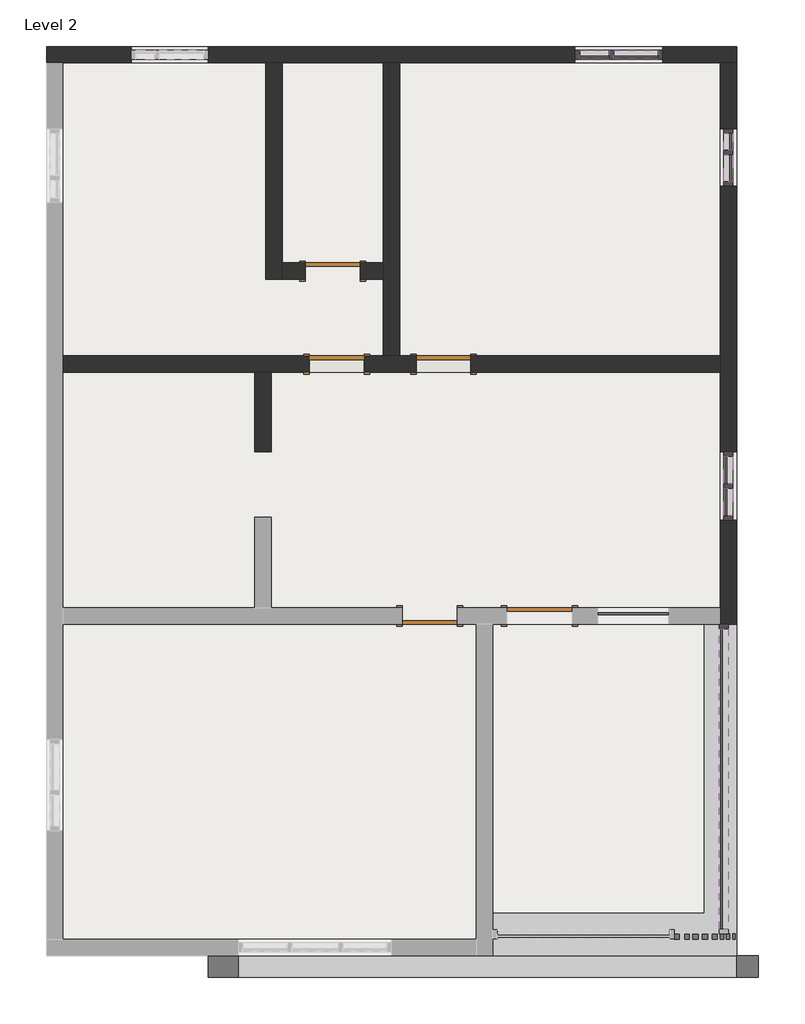
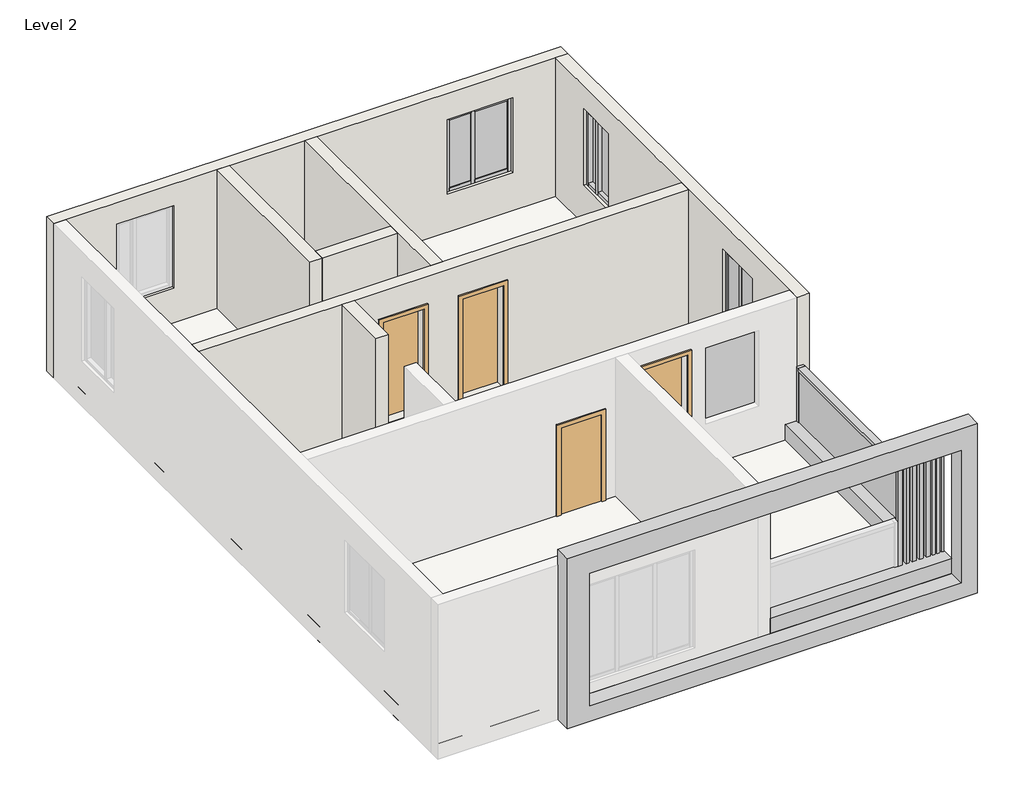
# One storey, part 2 of 2: 23 members, 8 plates, 7 walls, 5 doors, 1 proxy, 1 roof.
"""IFC4 building model written with IfcOpenShell, lengths in millimetres."""

from ifc_helpers import new_model, si_unit, frame, origin, place, context, project, spatial, polyline, outline, extrude, faceted_brep, transform, mapped, element, save
from components import generic_models_2_generic_models_2_9ece3dfc, door_a1484949, door_85036156, door_a90ba1ad, member_3f0e0172, member_dfe75557, member_af0bcaff, member_1d1a2070, member_a608d019, member_8d9b4452, member_2ab56126, member_a0c6f7ef, member_dc106669, member_53df7686, member_753b5246, member_6146d365, member_86c371d5, system_panel_glazed_3519d5a1, system_panel_glazed_546de4f7, system_panel_glazed_2f9bb5a6, system_panel_glazed_accf4d1c, system_panel_glazed_bfa5483a, system_panel_glazed_f170b818, system_panel_glazed_3acda581

model = new_model("IFC4")

# Units and contexts
model_context = context("Model", 3, world=origin())
ifc_project = project(units=[si_unit("LENGTHUNIT", "METRE", prefix="MILLI")], contexts=[model_context])

# Site, building, storey
site = spatial("IfcSite", under=ifc_project)
building = spatial("IfcBuilding", under=site)
storey = spatial("IfcBuildingStorey", under=building, Name="Level 2", Elevation=3048.0)

# Proxy
placement = place(None, origin())
generic_models_2_generic_models_2_shape = generic_models_2_generic_models_2_9ece3dfc(model_context)
element("IfcBuildingElementProxy", 1, Name="Generic Models 2 : Generic Models 2", ObjectType="Generic Models 2 : Generic Models 2", at=placement, inside=storey, context=model_context, shape_type="MappedRepresentation", body=[
    mapped(generic_models_2_generic_models_2_shape, transform((0.0, 0.0, 0.0), x_axis=(1.0, 0.0, 0.0), y_axis=(0.0, 1.0, 0.0), z_axis=(0.0, 0.0, 1.0))),
])

# Doors
door_shape = door_a1484949(model_context)
element("IfcDoor", 2, ObjectType="Single-Flush : 30\" x 80\"", at=placement, inside=storey, context=model_context, shape_type="MappedRepresentation", body=[
    mapped(door_shape, transform((-14545.6128107, -4291.2642965, 3048.0), x_axis=(1.0, 0.0, 0.0), y_axis=(0.0, 1.0, 0.0), z_axis=(0.0, 0.0, 1.0))),
])
element("IfcDoor", 3, ObjectType="Single-Flush : 30\" x 80\"", at=placement, inside=storey, context=model_context, shape_type="MappedRepresentation", body=[
    mapped(door_shape, transform((-14488.4628107, -5586.6642965, 3454.4), x_axis=(1.0, 0.0, 0.0), y_axis=(0.0, 1.0, 0.0), z_axis=(0.0, 0.0, 1.0))),
])
element("IfcDoor", 4, ObjectType="Single-Flush : 30\" x 80\"", at=placement, inside=storey, context=model_context, shape_type="MappedRepresentation", body=[
    mapped(door_shape, transform((-13193.0628107, -9091.8642965, 3048.0), x_axis=(-1.0, 0.0, 0.0), y_axis=(0.0, -1.0, 0.0), z_axis=(0.0, 0.0, 1.0))),
])
door_2_shape = door_85036156(model_context)
element("IfcDoor", 5, ObjectType="Single-Flush : 30\" x 80\"", at=placement, inside=storey, context=model_context, shape_type="MappedRepresentation", body=[
    mapped(door_2_shape, transform((-13002.5628107, -5586.6642965, 3403.6), x_axis=(-1.0, 0.0, 0.0), y_axis=(0.0, -1.0, 0.0), z_axis=(0.0, 0.0, 1.0))),
])
door_3_shape = door_a90ba1ad(model_context)
element("IfcDoor", 6, ObjectType="Single-Flush : 36\" x 84\"", at=placement, inside=storey, context=model_context, shape_type="MappedRepresentation", body=[
    mapped(door_3_shape, transform((-11669.0628107, -9091.8642965, 3556.0), x_axis=(-1.0, 0.0, 0.0), y_axis=(0.0, -1.0, 0.0), z_axis=(0.0, 0.0, 1.0))),
])

# Members
member_shape = member_3f0e0172(model_context)
element("IfcMember", 7, ObjectType="Rectangular Mullion : 2.5\" x 5\" rectangular", at=placement, inside=storey, context=model_context, shape_type="MappedRepresentation", body=[
    mapped(member_shape, transform((-10634.0128107, -1281.3642965, 5580.0830194), x_axis=(0.0, 0.0, 1.0), y_axis=(0.0, 1.0, 0.0), z_axis=(-1.0, 0.0, 0.0))),
])
element("IfcMember", 8, ObjectType="Rectangular Mullion : 2.5\" x 5\" rectangular", at=placement, inside=storey, context=model_context, shape_type="MappedRepresentation", body=[
    mapped(member_shape, transform((-10018.0628107, -1281.3642965, 4107.4786878), x_axis=(0.0, 0.0, -1.0), y_axis=(0.0, 1.0, 0.0), z_axis=(1.0, 0.0, 0.0))),
])
member_2_shape = member_dfe75557(model_context)
element("IfcMember", 9, ObjectType="Rectangular Mullion : 2.5\" x 5\" rectangular", at=placement, inside=storey, context=model_context, shape_type="MappedRepresentation", body=[
    mapped(member_2_shape, transform((-9040.1628107, -7250.3642965, 4008.2230499), x_axis=(0.0, 0.0, -1.0), y_axis=(1.0, 0.0, 0.0), z_axis=(0.0, -1.0, 0.0))),
])
element("IfcMember", 10, ObjectType="Rectangular Mullion : 2.5\" x 5\" rectangular", at=placement, inside=storey, context=model_context, shape_type="MappedRepresentation", body=[
    mapped(member_2_shape, transform((-9040.1628107, -7694.8642965, 4008.2230499), x_axis=(0.0, 0.0, -1.0), y_axis=(1.0, 0.0, 0.0), z_axis=(0.0, -1.0, 0.0))),
])
member_3_shape = member_af0bcaff(model_context)
element("IfcMember", 11, ObjectType="Rectangular Mullion : 2.5\" x 5\" rectangular", at=placement, inside=storey, context=model_context, shape_type="MappedRepresentation", body=[
    mapped(member_3_shape, transform((-9040.1628107, -7282.1142965, 4008.2230499), x_axis=(0.0, 1.0, 0.0), y_axis=(1.0, 0.0, 0.0), z_axis=(0.0, 0.0, -1.0))),
])
element("IfcMember", 12, ObjectType="Rectangular Mullion : 2.5\" x 5\" rectangular", at=placement, inside=storey, context=model_context, shape_type="MappedRepresentation", body=[
    mapped(member_2_shape, transform((-9040.1628107, -7313.8642965, 5591.2225485), x_axis=(0.0, 0.0, 1.0), y_axis=(1.0, 0.0, 0.0), z_axis=(0.0, 1.0, 0.0))),
])
element("IfcMember", 13, ObjectType="Rectangular Mullion : 2.5\" x 5\" rectangular", at=placement, inside=storey, context=model_context, shape_type="MappedRepresentation", body=[
    mapped(member_2_shape, transform((-9040.1628107, -6869.3642965, 5591.2225485), x_axis=(0.0, 0.0, 1.0), y_axis=(1.0, 0.0, 0.0), z_axis=(0.0, 1.0, 0.0))),
])
member_4_shape = member_1d1a2070(model_context)
element("IfcMember", 14, ObjectType="Rectangular Mullion : 2.5\" x 5\" rectangular", at=placement, inside=storey, context=model_context, shape_type="MappedRepresentation", body=[
    mapped(member_4_shape, transform((-9040.1628107, -6805.8642965, 4008.2230499), x_axis=(0.0, 1.0, 0.0), y_axis=(1.0, 0.0, 0.0), z_axis=(0.0, 0.0, -1.0))),
])
element("IfcMember", 15, ObjectType="Rectangular Mullion : 2.5\" x 5\" rectangular", at=placement, inside=storey, context=model_context, shape_type="MappedRepresentation", body=[
    mapped(member_4_shape, transform((-9040.1628107, -7758.3642965, 5591.2225485), x_axis=(0.0, -1.0, 0.0), y_axis=(1.0, 0.0, 0.0), z_axis=(0.0, 0.0, 1.0))),
])
member_5_shape = member_a608d019(model_context)
element("IfcMember", 16, ObjectType="Rectangular Mullion : 2.5\" x 5\" rectangular", at=placement, inside=storey, context=model_context, shape_type="MappedRepresentation", body=[
    mapped(member_5_shape, transform((-9040.1628107, -2608.5142965, 5637.0799904), x_axis=(0.0, 0.0, 1.0), y_axis=(-1.0, 0.0, 0.0), z_axis=(0.0, -1.0, 0.0))),
])
member_6_shape = member_8d9b4452(model_context)
element("IfcMember", 17, ObjectType="Rectangular Mullion : 2.5\" x 5\" rectangular", at=placement, inside=storey, context=model_context, shape_type="MappedRepresentation", body=[
    mapped(member_6_shape, transform((-9040.1628107, -3046.6642965, 5637.0799904), x_axis=(0.0, 0.0, 1.0), y_axis=(-1.0, 0.0, 0.0), z_axis=(0.0, -1.0, 0.0))),
])
member_7_shape = member_2ab56126(model_context)
element("IfcMember", 18, ObjectType="Rectangular Mullion : 2.5\" x 5\" rectangular", at=placement, inside=storey, context=model_context, shape_type="MappedRepresentation", body=[
    mapped(member_7_shape, transform((-9040.1628107, -2640.2642965, 4126.4819369), x_axis=(0.0, -1.0, 0.0), y_axis=(-1.0, 0.0, 0.0), z_axis=(0.0, 0.0, -1.0))),
])
element("IfcMember", 19, ObjectType="Rectangular Mullion : 2.5\" x 5\" rectangular", at=placement, inside=storey, context=model_context, shape_type="MappedRepresentation", body=[
    mapped(member_6_shape, transform((-9040.1628107, -2672.0142965, 4126.4819369), x_axis=(0.0, 0.0, -1.0), y_axis=(-1.0, 0.0, 0.0), z_axis=(0.0, 1.0, 0.0))),
])
element("IfcMember", 20, ObjectType="Rectangular Mullion : 2.5\" x 5\" rectangular", at=placement, inside=storey, context=model_context, shape_type="MappedRepresentation", body=[
    mapped(member_5_shape, transform((-9040.1628107, -2373.5642965, 4126.4819369), x_axis=(0.0, 0.0, -1.0), y_axis=(-1.0, 0.0, 0.0), z_axis=(0.0, 1.0, 0.0))),
])
member_8_shape = member_a0c6f7ef(model_context)
element("IfcMember", 21, ObjectType="Rectangular Mullion : 2.5\" x 5\" rectangular", at=placement, inside=storey, context=model_context, shape_type="MappedRepresentation", body=[
    mapped(member_8_shape, transform((-9040.1628107, -2310.0642965, 5637.0799904), x_axis=(0.0, 1.0, 0.0), y_axis=(-1.0, 0.0, 0.0), z_axis=(0.0, 0.0, 1.0))),
])
element("IfcMember", 22, ObjectType="Rectangular Mullion : 2.5\" x 5\" rectangular", at=placement, inside=storey, context=model_context, shape_type="MappedRepresentation", body=[
    mapped(member_8_shape, transform((-9040.1628107, -3110.1642965, 4126.4819369), x_axis=(0.0, -1.0, 0.0), y_axis=(-1.0, 0.0, 0.0), z_axis=(0.0, 0.0, -1.0))),
])
member_9_shape = member_dc106669(model_context)
element("IfcMember", 23, ObjectType="Rectangular Mullion : 2.5\" x 5\" rectangular", at=placement, inside=storey, context=model_context, shape_type="MappedRepresentation", body=[
    mapped(member_9_shape, transform((-11110.2628107, -1281.3642965, 5580.0830194), x_axis=(0.0, 0.0, 1.0), y_axis=(0.0, 1.0, 0.0), z_axis=(-1.0, 0.0, 0.0))),
])
member_10_shape = member_53df7686(model_context)
element("IfcMember", 24, ObjectType="Rectangular Mullion : 2.5\" x 5\" rectangular", at=placement, inside=storey, context=model_context, shape_type="MappedRepresentation", body=[
    mapped(member_10_shape, transform((-10665.7628107, -1281.3642965, 4107.4786878), x_axis=(-1.0, 0.0, 0.0), y_axis=(0.0, 1.0, 0.0), z_axis=(0.0, 0.0, -1.0))),
])
element("IfcMember", 25, ObjectType="Rectangular Mullion : 2.5\" x 5\" rectangular", at=placement, inside=storey, context=model_context, shape_type="MappedRepresentation", body=[
    mapped(member_9_shape, transform((-10697.5128107, -1281.3642965, 4107.4786878), x_axis=(0.0, 0.0, -1.0), y_axis=(0.0, 1.0, 0.0), z_axis=(1.0, 0.0, 0.0))),
])
member_11_shape = member_753b5246(model_context)
element("IfcMember", 26, ObjectType="Rectangular Mullion : 2.5\" x 5\" rectangular", at=placement, inside=storey, context=model_context, shape_type="MappedRepresentation", body=[
    mapped(member_11_shape, transform((-11173.7628107, -1281.3642965, 4107.4786878), x_axis=(-1.0, 0.0, 0.0), y_axis=(0.0, 1.0, 0.0), z_axis=(0.0, 0.0, -1.0))),
])
element("IfcMember", 27, ObjectType="Rectangular Mullion : 2.5\" x 5\" rectangular", at=placement, inside=storey, context=model_context, shape_type="MappedRepresentation", body=[
    mapped(member_11_shape, transform((-9954.5628107, -1281.3642965, 5580.0830194), x_axis=(1.0, 0.0, 0.0), y_axis=(0.0, 1.0, 0.0), z_axis=(0.0, 0.0, 1.0))),
])
member_12_shape = member_6146d365(model_context)
element("IfcMember", 28, ObjectType="Rectangular Mullion : 2.5\" x 5\" rectangular", at=placement, inside=storey, context=model_context, shape_type="MappedRepresentation", body=[
    mapped(member_12_shape, transform((-9103.6628107, -9206.1642965, 3436.1535444), x_axis=(0.0, 1.0, 0.0), y_axis=(1.0, 0.0, 0.0), z_axis=(0.0, 0.0, -1.0))),
])
member_13_shape = member_86c371d5(model_context)
element("IfcMember", 29, ObjectType="Rectangular Mullion : 2.5\" x 5\" rectangular", at=placement, inside=storey, context=model_context, shape_type="MappedRepresentation", body=[
    mapped(member_13_shape, transform((-9103.6628107, -9269.6642965, 4732.9155045), x_axis=(0.0, 0.0, 1.0), y_axis=(1.0, 0.0, 0.0), z_axis=(0.0, 1.0, 0.0))),
])

# Plates
system_panel_glazed_shape = system_panel_glazed_3519d5a1(model_context)
element("IfcPlate", 30, ObjectType="System Panel : Glazed", at=placement, inside=storey, context=model_context, shape_type="MappedRepresentation", body=[
    mapped(system_panel_glazed_shape, transform((-10360.9628107, -9091.8642965, 4193.7740011), x_axis=(1.0, 0.0, 0.0), y_axis=(0.0, 1.0, 0.0), z_axis=(0.0, 0.0, 1.0))),
])
system_panel_glazed_2_shape = system_panel_glazed_546de4f7(model_context)
element("IfcPlate", 31, ObjectType="System Panel : Glazed", at=placement, inside=storey, context=model_context, shape_type="MappedRepresentation", body=[
    mapped(system_panel_glazed_2_shape, transform((-9040.1628107, -7504.3642965, 4071.7230499), x_axis=(0.0, 1.0, 0.0), y_axis=(-1.0, 0.0, 0.0), z_axis=(0.0, 0.0, 1.0))),
])
element("IfcPlate", 32, ObjectType="System Panel : Glazed", at=placement, inside=storey, context=model_context, shape_type="MappedRepresentation", body=[
    mapped(system_panel_glazed_2_shape, transform((-9040.1628107, -7059.8642965, 4071.7230499), x_axis=(0.0, 1.0, 0.0), y_axis=(-1.0, 0.0, 0.0), z_axis=(0.0, 0.0, 1.0))),
])
system_panel_glazed_3_shape = system_panel_glazed_2f9bb5a6(model_context)
element("IfcPlate", 33, ObjectType="System Panel : Glazed", at=placement, inside=storey, context=model_context, shape_type="MappedRepresentation", body=[
    mapped(system_panel_glazed_3_shape, transform((-9040.1628107, -2491.0392965, 4189.9819369), x_axis=(0.0, -1.0, 0.0), y_axis=(1.0, 0.0, 0.0), z_axis=(0.0, 0.0, 1.0))),
])
system_panel_glazed_4_shape = system_panel_glazed_accf4d1c(model_context)
element("IfcPlate", 34, ObjectType="System Panel : Glazed", at=placement, inside=storey, context=model_context, shape_type="MappedRepresentation", body=[
    mapped(system_panel_glazed_4_shape, transform((-9040.1628107, -2859.3392965, 4189.9819369), x_axis=(0.0, -1.0, 0.0), y_axis=(1.0, 0.0, 0.0), z_axis=(0.0, 0.0, 1.0))),
])
system_panel_glazed_5_shape = system_panel_glazed_bfa5483a(model_context)
element("IfcPlate", 35, ObjectType="System Panel : Glazed", at=placement, inside=storey, context=model_context, shape_type="MappedRepresentation", body=[
    mapped(system_panel_glazed_5_shape, transform((-10326.0378107, -1281.3642965, 4170.9786878), x_axis=(-1.0, 0.0, 0.0), y_axis=(0.0, -1.0, 0.0), z_axis=(0.0, 0.0, 1.0))),
])
system_panel_glazed_6_shape = system_panel_glazed_f170b818(model_context)
element("IfcPlate", 36, ObjectType="System Panel : Glazed", at=placement, inside=storey, context=model_context, shape_type="MappedRepresentation", body=[
    mapped(system_panel_glazed_6_shape, transform((-10903.8878107, -1281.3642965, 4170.9786878), x_axis=(-1.0, 0.0, 0.0), y_axis=(0.0, -1.0, 0.0), z_axis=(0.0, 0.0, 1.0))),
])
system_panel_glazed_7_shape = system_panel_glazed_3acda581(model_context)
element("IfcPlate", 37, ObjectType="System Panel : Glazed", at=placement, inside=storey, context=model_context, shape_type="MappedRepresentation", body=[
    mapped(system_panel_glazed_7_shape, transform((-9103.6628107, -11358.8142965, 3499.6535444), x_axis=(0.0, 1.0, 0.0), y_axis=(-1.0, 0.0, 0.0), z_axis=(0.0, 0.0, 1.0))),
])

# Roof
element("IfcRoof", 38, ObjectType="Generic - 12\"", at=placement, inside=storey, context=model_context, shape_type="SweptSolid", body=[
    extrude(outline(polyline([(-18527.0628107, -1167.0642965), (-8925.8628107, -1167.0642965), (-8925.8628107, -13816.2642965), (-18527.0628107, -13816.2642965), (-18527.0628107, -1167.0642965)])), frame((0.0, 0.0, 3048.0), z_axis=(0.0, 0.0, 1.0), x_axis=(1.0, 0.0, 0.0)), (0.0, 0.0, 1.0), 304.8),
])

# Walls
element("IfcWall", 39, ObjectType="9\"", at=placement, inside=storey, context=model_context, shape_type="Brep", body=[
    faceted_brep([(-18527.0628107, -1395.6642965, 3048.0), (-18298.4628107, -1395.6642965, 3048.0), (-15479.0628107, -1395.6642965, 3048.0), (-15250.4628107, -1395.6642965, 3048.0), (-13840.7628107, -1395.6642965, 3048.0), (-13612.1628107, -1395.6642965, 3048.0), (-9154.4628107, -1395.6642965, 3048.0), (-8925.8628107, -1395.6642965, 3048.0), (-8925.8628107, -1395.6642965, 6096.0), (-9154.4628107, -1395.6642965, 6096.0), (-13612.1628107, -1395.6642965, 6096.0), (-13840.7628107, -1395.6642965, 6096.0), (-15250.4628107, -1395.6642965, 6096.0), (-15479.0628107, -1395.6642965, 6096.0), (-18298.4628107, -1395.6642965, 6096.0), (-18527.0628107, -1395.6642965, 6096.0), (-9954.5628107, -1395.6642965, 5580.0830194), (-9954.5628107, -1395.6642965, 4107.4786878), (-11173.7628107, -1395.6642965, 4107.4786878), (-11173.7628107, -1395.6642965, 5580.0830194), (-17345.9628107, -1395.6642965, 4034.7127427), (-17345.9628107, -1395.6642965, 5669.0676645), (-16279.1628107, -1395.6642965, 5669.0676645), (-16279.1628107, -1395.6642965, 4034.7127427), (-8925.8628107, -1167.0642965, 3048.0), (-18527.0628107, -1167.0642965, 3048.0), (-18527.0628107, -1167.0642965, 6096.0), (-8925.8628107, -1167.0642965, 6096.0), (-9954.5628107, -1167.0642965, 4107.4786878), (-9954.5628107, -1167.0642965, 5580.0830194), (-11173.7628107, -1167.0642965, 5580.0830194), (-11173.7628107, -1167.0642965, 4107.4786878), (-17345.9628107, -1167.0642965, 5669.0676645), (-17345.9628107, -1167.0642965, 4034.7127427), (-16279.1628107, -1167.0642965, 4034.7127427), (-16279.1628107, -1167.0642965, 5669.0676645)], [[[0, 1, 2, 3, 4, 5, 6, 7, 8, 9, 10, 11, 12, 13, 14, 15], [16, 17, 18, 19], [20, 21, 22, 23]], [[24, 25, 26, 27], [28, 29, 30, 31], [32, 33, 34, 35]], [[7, 6, 5, 4, 3, 2, 1, 0, 25, 24]], [[15, 14, 13, 12, 11, 10, 9, 8, 27, 26]], [[8, 7, 24, 27]], [[0, 15, 26, 25]], [[16, 29, 28, 17]], [[29, 16, 19, 30]], [[30, 19, 18, 31]], [[17, 28, 31, 18]], [[20, 33, 32, 21]], [[21, 32, 35, 22]], [[22, 35, 34, 23]], [[33, 20, 23, 34]]]),
])
element("IfcWall", 40, ObjectType="9\"", at=placement, inside=storey, context=model_context, shape_type="Brep", body=[
    faceted_brep([(-9154.4628107, -1395.6642965, 3048.0), (-9154.4628107, -5472.3642965, 3048.0), (-9154.4628107, -5700.9642965, 3048.0), (-9154.4628107, -8977.5642965, 3048.0), (-9154.4628107, -9206.1642965, 3048.0), (-9154.4628107, -9206.1642965, 6096.0), (-9154.4628107, -8977.5642965, 6096.0), (-9154.4628107, -5700.9642965, 6096.0), (-9154.4628107, -5472.3642965, 6096.0), (-9154.4628107, -1395.6642965, 6096.0), (-9154.4628107, -7758.3642965, 5591.2225485), (-9154.4628107, -7758.3642965, 4008.2230499), (-9154.4628107, -6805.8642965, 4008.2230499), (-9154.4628107, -6805.8642965, 5591.2225485), (-9154.4628107, -2310.0642965, 4126.4819369), (-9154.4628107, -2310.0642965, 5637.0799904), (-9154.4628107, -3110.1642965, 5637.0799904), (-9154.4628107, -3110.1642965, 4126.4819369), (-8925.8628107, -9206.1642965, 3048.0), (-8925.8628107, -1395.6642965, 3048.0), (-8925.8628107, -1395.6642965, 6096.0), (-8925.8628107, -9206.1642965, 6096.0), (-8925.8628107, -7758.3642965, 4008.2230499), (-8925.8628107, -7758.3642965, 5591.2225485), (-8925.8628107, -6805.8642965, 5591.2225485), (-8925.8628107, -6805.8642965, 4008.2230499), (-8925.8628107, -2310.0642965, 5637.0799904), (-8925.8628107, -2310.0642965, 4126.4819369), (-8925.8628107, -3110.1642965, 4126.4819369), (-8925.8628107, -3110.1642965, 5637.0799904)], [[[0, 1, 2, 3, 4, 5, 6, 7, 8, 9], [10, 11, 12, 13], [14, 15, 16, 17]], [[18, 19, 20, 21], [22, 23, 24, 25], [26, 27, 28, 29]], [[4, 3, 2, 1, 0, 19, 18]], [[9, 8, 7, 6, 5, 21, 20]], [[0, 9, 20, 19]], [[5, 4, 18, 21]], [[10, 23, 22, 11]], [[23, 10, 13, 24]], [[24, 13, 12, 25]], [[11, 22, 25, 12]], [[14, 27, 26, 15]], [[15, 26, 29, 16]], [[16, 29, 28, 17]], [[27, 14, 17, 28]]]),
])
element("IfcWall", 41, ObjectType="9\"", at=placement, inside=storey, context=model_context, shape_type="Brep", body=[
    faceted_brep([(-9154.4628107, -5472.3642965, 3048.0), (-13612.1628107, -5472.3642965, 3048.0), (-13840.7628107, -5472.3642965, 3048.0), (-18298.4628107, -5472.3642965, 3048.0), (-18298.4628107, -5472.3642965, 6096.0), (-13840.7628107, -5472.3642965, 6096.0), (-13612.1628107, -5472.3642965, 6096.0), (-9154.4628107, -5472.3642965, 6096.0), (-13383.5628107, -5472.3642965, 3403.6), (-12621.5628107, -5472.3642965, 3403.6), (-12621.5628107, -5472.3642965, 5435.6), (-13383.5628107, -5472.3642965, 5435.6), (-14869.4628107, -5472.3642965, 3454.4), (-14107.4628107, -5472.3642965, 3454.4), (-14107.4628107, -5472.3642965, 5486.4), (-14869.4628107, -5472.3642965, 5486.4), (-18298.4628107, -5700.9642965, 3048.0), (-15631.4628107, -5700.9642965, 3048.0), (-15402.8628107, -5700.9642965, 3048.0), (-9154.4628107, -5700.9642965, 3048.0), (-9154.4628107, -5700.9642965, 6096.0), (-15402.8628107, -5700.9642965, 6096.0), (-15631.4628107, -5700.9642965, 6096.0), (-18298.4628107, -5700.9642965, 6096.0), (-12621.5628107, -5700.9642965, 3403.6), (-13383.5628107, -5700.9642965, 3403.6), (-13383.5628107, -5700.9642965, 5435.6), (-12621.5628107, -5700.9642965, 5435.6), (-14107.4628107, -5700.9642965, 3454.4), (-14869.4628107, -5700.9642965, 3454.4), (-14869.4628107, -5700.9642965, 5486.4), (-14107.4628107, -5700.9642965, 5486.4)], [[[0, 1, 2, 3, 4, 5, 6, 7], [8, 9, 10, 11], [12, 13, 14, 15]], [[16, 17, 18, 19, 20, 21, 22, 23], [24, 25, 26, 27], [28, 29, 30, 31]], [[3, 2, 1, 0, 19, 18, 17, 16]], [[7, 6, 5, 4, 23, 22, 21, 20]], [[0, 7, 20, 19]], [[4, 3, 16, 23]], [[24, 9, 8, 25]], [[25, 8, 11, 26]], [[26, 11, 10, 27]], [[9, 24, 27, 10]], [[13, 12, 29, 28]], [[14, 13, 28, 31]], [[15, 14, 31, 30]], [[12, 15, 30, 29]]]),
])
element("IfcWall", 42, ObjectType="9\"", at=placement, inside=storey, context=model_context, shape_type="Brep", body=[
    faceted_brep([(-13612.1628107, -5472.3642965, 3048.0), (-13612.1628107, -1395.6642965, 3048.0), (-13612.1628107, -1395.6642965, 6096.0), (-13612.1628107, -5472.3642965, 6096.0), (-13840.7628107, -5472.3642965, 3048.0), (-13840.7628107, -5472.3642965, 6096.0), (-13840.7628107, -4405.5642965, 6096.0), (-13840.7628107, -4176.9642965, 6096.0), (-13840.7628107, -1395.6642965, 6096.0), (-13840.7628107, -1395.6642965, 3048.0), (-13840.7628107, -4176.9642965, 3048.0), (-13840.7628107, -4405.5642965, 3048.0)], [[[0, 1, 2, 3]], [[4, 5, 6, 7, 8, 9, 10, 11]], [[1, 0, 4, 11, 10, 9]], [[3, 2, 8, 7, 6, 5]], [[0, 3, 5, 4]], [[2, 1, 9, 8]]]),
])
element("IfcWall", 43, ObjectType="9\"", at=placement, inside=storey, context=model_context, shape_type="Brep", body=[
    faceted_brep([(-15479.0628107, -1395.6642965, 3048.0), (-15479.0628107, -4405.5642965, 3048.0), (-15479.0628107, -4405.5642965, 6096.0), (-15479.0628107, -1395.6642965, 6096.0), (-15250.4628107, -1395.6642965, 3048.0), (-15250.4628107, -1395.6642965, 6096.0), (-15250.4628107, -4176.9642965, 6096.0), (-15250.4628107, -4405.5642965, 6096.0), (-15250.4628107, -4405.5642965, 3048.0), (-15250.4628107, -4176.9642965, 3048.0)], [[[0, 1, 2, 3]], [[4, 5, 6, 7, 8, 9]], [[1, 0, 4, 9, 8]], [[3, 2, 7, 6, 5]], [[0, 3, 5, 4]], [[2, 1, 8, 7]]]),
])
element("IfcWall", 44, ObjectType="9\"", at=placement, inside=storey, context=model_context, shape_type="SweptSolid", body=[
    extrude(outline(polyline([(5080.0, -14164.6128107), (3048.0, -14164.6128107), (3048.0, -13840.7628107), (6096.0, -13840.7628107), (6096.0, -15250.4628107), (3048.0, -15250.4628107), (3048.0, -14926.6128107), (5080.0, -14926.6128107), (5080.0, -14164.6128107)])), frame((0.0, -4405.5642965, 0.0), z_axis=(0.0, 1.0, 0.0), x_axis=(0.0, 0.0, 1.0)), (0.0, 0.0, 1.0), 228.6),
])
element("IfcWall", 45, ObjectType="9\"", at=placement, inside=storey, context=model_context, shape_type="SweptSolid", body=[
    extrude(outline(polyline([(-15631.4628107, -6805.8642965), (-15631.4628107, -5700.9642965), (-15402.8628107, -5700.9642965), (-15402.8628107, -6805.8642965), (-15631.4628107, -6805.8642965)])), frame((0.0, 0.0, 3048.0), z_axis=(0.0, 0.0, 1.0), x_axis=(1.0, 0.0, 0.0)), (0.0, 0.0, 1.0), 3048.0),
])

save(model, "model.ifc")

# Revit data of these elements
# Type "Single-Flush : 30\" x 80\""
#   Type Mark = "5"
#   Construction Type Id = "MDOOR"
#   Assembly Code = "C1020"
#   Analytic Construction = "Metal"
#   Thickness = 0' - 2"
#   Heat Transfer Coefficient (U) = 0.651978 BTU/(h·ft²·°F)
#   Height = 6' - 8"
#   Trim Projection Ext = 0' - 1"
#   Trim Projection Int = 0' - 1"
#   Trim Width = 0' - 3"
#   Width = 2' - 6"
#   Define Thermal Properties by = 1
#   Define Thermal Properties by = 1
#   Door Material = Door - Panel
#   Frame Material = Door - Frame
#   Visual Light Transmittance = 0
#   Solar Heat Gain Coefficient = 0
#   Function = (empty or 0)
#   Wall Closure = (empty or 0)
# Type "Single-Flush : 36\" x 84\""
#   Type Mark = "1"
#   Construction Type Id = "MDOOR"
#   Assembly Code = "C1020"
#   Analytic Construction = "Metal"
#   Thickness = 0' - 2"
#   Heat Transfer Coefficient (U) = 0.651978 BTU/(h·ft²·°F)
#   Height = 7' - 0"
#   Trim Projection Ext = 0' - 1"
#   Trim Projection Int = 0' - 1"
#   Trim Width = 0' - 3"
#   Width = 3' - 0"
#   Define Thermal Properties by = 1
#   Define Thermal Properties by = 1
#   Door Material = Door - Panel
#   Frame Material = Door - Frame
#   Visual Light Transmittance = 0
#   Solar Heat Gain Coefficient = 0
#   Function = (empty or 0)
#   Wall Closure = (empty or 0)
# Type "Rectangular Mullion : 2.5\" x 5\" rectangular"
#   built-in parameter 1007304 = 0.416667 (stored number, unit not read)
#   built-in parameter 1007301 = 0.104167 (stored number, unit not read)
#   built-in parameter 1007300 = 0.104167 (stored number, unit not read)
# Type "System Panel : Glazed"
#   Construction Type Id = "GSP4R"
#   Analytic Construction = "1/8 in Pilkington single glazing"
#   Visual Light Transmittance = 0.9
#   Solar Heat Gain Coefficient = 0.86
#   Heat Transfer Coefficient (U) = 1.18115 BTU/(h·ft²·°F)
#   Define Thermal Properties by = 1
# Type "Generic - 12\""
#   Assembly Code = "B1020"
#   Layers, outside or top first: 1' - 0" no material (function 1)
# Type "9\""
#   Assembly Code = "B2010"
#   Layers, outside or top first: 0' - 9" no material (function 1)
# Element 1 (IfcBuildingElementProxy, "Generic Models 2 : Generic Models 2")
#   Phase Created = New Construction
# Elements 2, 3, 4, 5 (IfcDoor, "Single-Flush : 30\" x 80\"")
#   Phase Created = New Construction
#   Materials on its faces: "Door - Frame", "Door - Panel"
# Element 6 (IfcDoor, "Single-Flush : 36\" x 84\"")
#   Phase Created = New Construction
#   Materials on its faces: "Door - Frame", "Door - Panel"
# Elements 7, 8, 9, 10, 11, 12, 13, 14, 15, 16, 17, 18, 19, 20, 21, 22, 23, 24, 25, 26, 27, 28, 29 (IfcMember, "Rectangular Mullion : 2.5\" x 5\" rectangular")
#   Phase Created = New Construction
#   Materials on its faces: "Aluminum"
# Elements 30, 31, 32, 33, 34, 35, 36, 37 (IfcPlate, "System Panel : Glazed")
#   Phase Created = New Construction
#   Materials on its faces: "Glass"
# Element 38 (IfcRoof, "Generic - 12\"")
#   built-in parameter 1001705 = 11 (stored number, unit not read)
#   built-in parameter 1001710 = 33615
#   Phase Created = New Construction
#   Materials on its faces: "Default Roof"
# Elements 39, 40, 41, 42, 43, 44, 45 (IfcWall, "9\"")
#   Top Offset = 0' - 0"
#   Base Offset = 0' - 0"
#   Unconnected Height = 10' - 0"
#   wall height = 10' - 0"
#   Phase Created = New Construction
#   Base Constraint = Level 2
#   Materials on its faces: "Default Wall"
# Materials
#   "Door - Panel": class "Wood", colour RGB 210 159 95, transparency 0, Cost = 0
#   "Door - Frame": colour RGB 118 70 51, transparency 0, Cost = 0
#   "Aluminum": class "Metal", colour RGB 247 247 247, transparency 0, Description = "Aluminum 6061", Cost = 0
#   "Glass": class "Glass", colour RGB 0 128 192, transparency 0.75, Description = "Soda Lime Glass", Cost = 0
#   "Default Roof": colour RGB 88 101 114, transparency 0, Cost = 0
#   "Default Wall": colour RGB 128 128 128, transparency 0, Cost = 0
